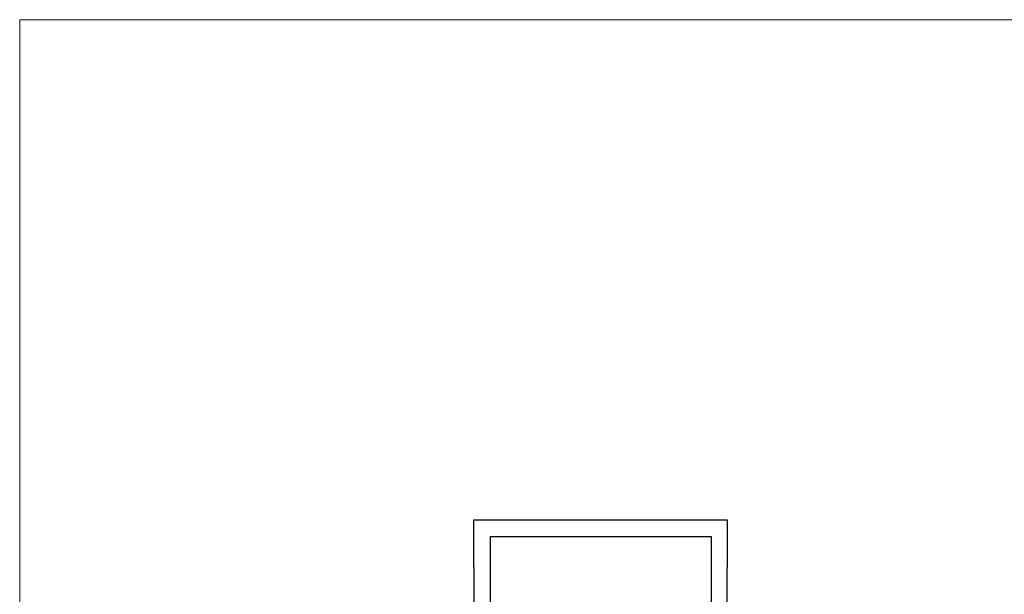
# Model space of a CAD drawing. Units: inches. Extents: x 1901 to 2863, y 888 to 2433.
# Tile 63 of 91: x 1901 to 2169, y 2277 to 2433. Entities that reach past the tile are written whole.
import ezdxf

# ---------------------------------------------------------------- set-up
doc = ezdxf.new("R2010")
doc.units = ezdxf.units.IN
doc.layers.add('A-FLOR-FIXT', color=9, linetype='Continuous', lineweight=18)
doc.layers.add('A-FLOR-HRAL', color=41, linetype='Continuous', lineweight=25)

msp = doc.modelspace()

# ---------------------------------------------------------------- linework, layer by layer
at = {"layer": 'A-FLOR-FIXT'}
msp.add_lwpolyline([(1901.45, 2433.12), (2863.43, 2433.12), (2863.43, 961.82), (1901.45, 961.82)], close=True, dxfattribs=at)
at = {"layer": 'A-FLOR-HRAL'}
for p, q in [((2024.93, 2292.63), (2024.93, 2297.13)), ((2024.93, 2297.13), (2093.82, 2297.13)), ((2093.82, 2297.13), (2093.82, 2284.13)), ((2024.93, 2284.13), (2024.93, 2292.63)), ((2029.43, 2219.63), (2029.43, 2292.63)), ((2029.43, 2292.63), (2089.43, 2292.63)), ((2089.43, 2292.63), (2089.43, 2279.63)), ((2024.93, 2284.13), (2024.93, 2219.63)), ((2093.82, 2279.63), (2093.82, 2284.13)), ((2089.43, 2279.63), (2089.43, 2274.13)), ((2093.82, 2274.13), (2093.82, 2279.63))]:
    msp.add_line(p, q, dxfattribs=at)

doc.saveas('drawing.dxf')
